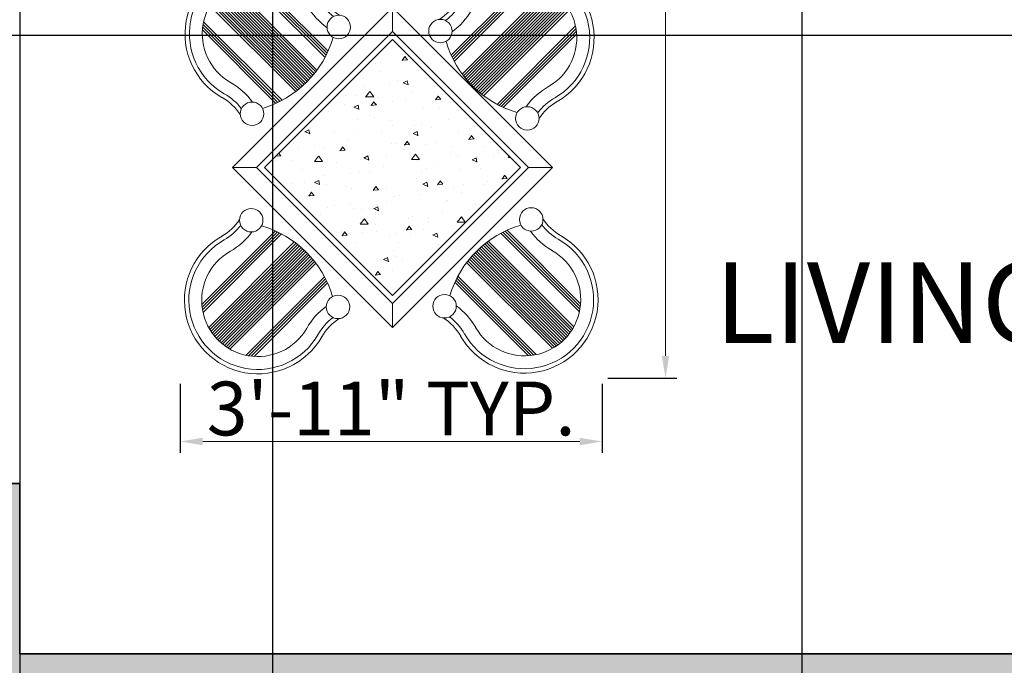
# Model space of a CAD drawing. Units: inches. Extents: x 2696 to 3240, y 1564 to 2310.
# Tile 23 of 76: x 2755 to 2864, y 1910 to 1982. Entities that reach past the tile are written whole.
import ezdxf

# ---------------------------------------------------------------- set-up
doc = ezdxf.new("R2010")
doc.units = ezdxf.units.IN
for name, color, linetype, lineweight in [('A-ANNO-DIMS', 3, 'Continuous', 18), ('A-AREA-IDEN', 7, 'Continuous', 18), ('A-FURN', 251, 'Continuous', 13), ('A-WALL', 7, 'Continuous', 35), ('A-WALL-PATT', 9, 'Continuous', 13), ('WINDOW', 2, 'Continuous', 18)]:
    doc.layers.add(name, color=color, linetype=linetype, lineweight=lineweight)
doc.styles.add('TIMES NEW', font='times.ttf')
doc.styles.add('YQ_DIM', font='SUPEROS.SHX', dxfattribs={"width": 0.8, "bigfont": 'HZDX.SHX'})
doc.dimstyles.new('Siddhuu', dxfattribs={"dimtxt": 6, "dimasz": 2.5, "dimexe": 1.25, "dimexo": 0.625, "dimtad": 1, "dimdec": 1, "dimlunit": 4, "dimtxsty": 'TIMES NEW', "dimcen": 2.5, "dimclrd": 256, "dimclre": 1, "dimclrt": 7, "dimadec": 0, "dimazin": 0, "dimtfac": 1, "dimtdec": 1, "dimtmove": 0, "dimatfit": 3, "dimfxl": 1, "dimtolj": 1, "dimlwd": -1, "dimarcsym": 0})

# ---------------------------------------------------------------- blocks, each defined once
blk = doc.blocks.new('WD_WIN4')
for p, q in [((-0.5, 0.5), (0.5, 0.5)), ((-0.5, 0.12), (0.5, 0.12)), ((-0.5, -0.12), (0.5, -0.12)), ((-0.5, -0.5), (0.5, -0.5))]:
    blk.add_line(p, q)
blk = doc.blocks.new('DINING-SET-4')
h = blk.add_hatch()
h.set_pattern_fill('AR-CONC,_O', color=256, scale=0.03156, angle=135)
h.set_pattern_definition([(185, (694.1166, -47.9622), (-3.709933, 4.421326), [0.60121, -6.613307]), (130, (694.1166, -47.962), (-3.47714, -5.050095), [0.48097, -5.290645]), (235.451, (693.8074, -47.594), (-7.187067, -0.628735), [0.51095, -5.620443]), (181.1842, (692.983, -49.096), (-5.11118, 6.98761), [0.90181, -9.91996]), (231.6356, (692.557, -48.514), (-10.81945, -0.22364), [0.76642, -8.43066]), (126.184, (692.983, -49.096), (-10.81945, -0.22362), [0.72145, -7.93597]), (156, (692.6995, -48.2457), (-1.10128, 5.66559), [0.60121, -6.613307]), (101, (692.6995, -48.2457), (-5.48951, -2.73116), [0.48097, -5.290645]), (206.4514, (692.608, -47.7735), (-6.590787, 2.93441), [0.51095, -5.620443]), (172.5, (694.1166, -47.9622), (-1.955854, -1.8180035), [0, -5.226516, 0, -5.370807, 0, -5.310686]), (142.5, (694.1166, -47.9622), (-3.726774, -0.744482), [0, -3.062161, 0, -5.106274, 0, -2.024073]), (102.5, (695.3806, -49.2263), (-2.8979947, 3.15368), [0, -2.004032, 0, -6.25258, 0, -8.296694]), (92.5, (695.9475, -49.793), (-3.873065, 2.73823), [0, -2.605242, 0, -4.152355, 0, -5.891855])])
h.paths.add_polyline_path([(23.22, 8.74), (37.5, 23.02), (23.22, 37.31), (8.94, 23.02)])
for p, q in [((15.69, 35.33), (6.93, 44.09)), ((15.81, 35.56), (7.22, 44.15)), ((15.92, 35.79), (7.52, 44.19)), ((16.03, 36.02), (7.83, 44.22)), ((14.19, 33.15), (4.42, 42.91)), ((14.34, 33.33), (4.62, 43.06)), ((14.5, 33.52), (4.82, 43.2)), ((14.65, 33.71), (5.03, 43.33)), ((14.79, 33.91), (5.25, 43.45)), ((29.77, 35.57), (37.97, 43.77)), ((29.88, 35.34), (38.28, 43.74)), ((29.99, 35.11), (38.58, 43.7)), ((30.11, 34.88), (38.86, 43.64)), ((31, 33.46), (40.55, 43.01)), ((31.15, 33.26), (40.76, 42.88)), ((13.17, 32.12), (3.39, 41.89)), ((13.35, 32.28), (3.55, 42.08)), ((13.52, 32.45), (3.71, 42.26)), ((13.69, 32.62), (3.88, 42.43)), ((13.86, 32.79), (4.05, 42.6)), ((14.03, 32.97), (4.24, 42.76)), ((31.3, 33.07), (40.97, 42.75)), ((31.45, 32.88), (41.18, 42.61)), ((31.61, 32.7), (41.37, 42.46)), ((31.77, 32.52), (41.56, 42.31)), ((31.93, 32.34), (41.74, 42.15)), ((32.1, 32.17), (41.92, 41.98)), ((32.27, 32), (42.09, 41.81)), ((12.42, 31.5), (2.84, 41.08)), ((12.61, 31.65), (2.97, 41.3)), ((12.8, 31.8), (3.1, 41.5)), ((12.99, 31.96), (3.24, 41.7)), ((23.22, 38.2), (23.22, 40.88)), ((32.45, 31.83), (42.25, 41.63)), ((32.63, 31.67), (42.4, 41.45)), ((32.81, 31.51), (42.55, 41.25)), ((32.99, 31.35), (42.69, 41.05)), ((33.18, 31.2), (42.83, 40.85)), ((33.38, 31.05), (42.96, 40.63)), ((10.44, 30.3), (2.05, 38.7)), ((10.67, 30.41), (2.09, 39)), ((10.9, 30.53), (2.15, 39.28)), ((34.9, 30.08), (43.65, 38.83)), ((35.12, 29.96), (43.7, 38.55)), ((10.21, 30.19), (2.02, 38.38)), ((35.35, 29.85), (43.75, 38.25)), ((35.58, 29.74), (43.78, 37.94)), ((8.05, 23.02), (5.37, 23.02)), ((38.4, 23.02), (41.07, 23.02)), ((10.15, 15.95), (1.95, 7.75)), ((10.38, 15.84), (1.98, 7.44)), ((10.61, 15.73), (2.02, 7.14)), ((10.84, 15.61), (2.08, 6.86)), ((35.33, 15.7), (44.08, 6.94)), ((35.55, 15.81), (44.14, 7.23)), ((35.78, 15.93), (44.18, 7.52)), ((36.01, 16.03), (44.21, 7.83)), ((12.26, 14.72), (2.71, 5.17)), ((12.46, 14.57), (2.84, 4.95)), ((12.65, 14.42), (2.97, 4.75)), ((33.33, 14.35), (43.05, 4.63)), ((33.51, 14.5), (43.19, 4.83)), ((33.7, 14.65), (43.32, 5.04)), ((33.9, 14.8), (43.45, 5.25)), ((12.83, 14.27), (3.11, 4.54)), ((13.02, 14.11), (3.26, 4.35)), ((13.2, 13.95), (3.41, 4.16)), ((13.38, 13.78), (3.57, 3.98)), ((13.55, 13.62), (3.74, 3.8)), ((13.72, 13.45), (3.91, 3.63)), ((13.89, 13.27), (4.09, 3.47)), ((32.27, 13.35), (42.07, 3.55)), ((32.44, 13.53), (42.25, 3.72)), ((32.61, 13.7), (42.42, 3.89)), ((32.78, 13.87), (42.59, 4.06)), ((32.96, 14.03), (42.75, 4.24)), ((33.14, 14.19), (42.9, 4.43)), ((14.05, 13.09), (4.27, 3.32)), ((14.21, 12.91), (4.47, 3.17)), ((14.36, 12.72), (4.67, 3.03)), ((14.52, 12.54), (4.87, 2.89)), ((14.67, 12.34), (5.08, 2.76)), ((31.49, 12.43), (41.08, 2.85)), ((31.64, 12.62), (41.29, 2.97)), ((31.8, 12.81), (41.5, 3.11)), ((31.95, 12.99), (41.69, 3.25)), ((32.11, 13.18), (41.89, 3.4)), ((15.64, 10.82), (6.89, 2.07)), ((15.75, 10.6), (7.17, 2.02)), ((15.87, 10.37), (7.47, 1.97)), ((15.98, 10.14), (7.78, 1.94)), ((30.18, 10.22), (38.38, 2.03)), ((30.29, 10.45), (38.69, 2.06)), ((30.41, 10.68), (38.99, 2.1)), ((30.52, 10.91), (39.27, 2.15)), ((23.22, 7.85), (23.22, 5.17))]:
    blk.add_line(p, q)
for points in [[(41.07, 23.02), (23.22, 40.88), (5.37, 23.02), (23.22, 5.17)], [(38.4, 23.02), (23.22, 38.2), (8.05, 23.02), (23.22, 7.85)], [(37.5, 23.02), (23.22, 37.31), (8.94, 23.02), (23.22, 8.74)]]:
    blk.add_lwpolyline(points, close=True)
for centre in [(17.23, 38.71), (28.57, 38.26), (7.55, 29.03), (38.27, 28.51), (7.46, 17.15), (38.7, 17.23), (29.03, 7.55), (17.14, 7.47)]:
    blk.add_circle(centre, 1.31)
for centre, radius, start, end in [((8.28, 37.96), 8.21, 29.1881, 240.1532), ((8.28, 37.96), 7.72, 29.1881, 240.1532), ((37.51, 37.51), 8.21, 299.8468, 150.8119), ((37.51, 37.51), 7.72, 299.8468, 150.8119), ((8.28, 37.96), 6.28, 29.2752, 240.1505), ((37.51, 37.51), 6.28, 299.8495, 150.7248), ((20.45, 44.88), 5.79, 210.1015, 236.9513), ((20.45, 44.88), 7.72, 209.8594, 234.0675), ((20.45, 44.88), 6.28, 210.1015, 232.6572), ((25.34, 44.43), 5.79, 303.0487, 329.8985), ((25.34, 44.43), 6.28, 307.3428, 329.8985), ((25.34, 44.43), 7.72, 305.9325, 330.1406), ((5.4, 40.81), 11.66, 286.5158, 343.8317), ((40.4, 40.36), 11.66, 196.1683, 253.4842), ((1.37, 25.79), 7.72, 36.1055, 60.6071), ((44.43, 25.34), 7.72, 119.3929, 143.8945), ((1.37, 25.79), 5.79, 32.6748, 60.7093), ((1.37, 25.79), 6.28, 37.2611, 60.7093), ((44.43, 25.34), 6.28, 119.2907, 142.7389), ((44.43, 25.34), 5.79, 119.2907, 147.3252), ((1.29, 20.38), 5.79, 300.1015, 326.9513), ((1.29, 20.38), 6.28, 300.1015, 322.6572), ((5.36, 5.32), 11.66, 16.5158, 73.8317), ((40.8, 5.4), 11.66, 106.1683, 163.4842), ((44.87, 20.46), 6.28, 217.3428, 239.8985), ((44.87, 20.46), 5.79, 213.0487, 239.8985), ((1.29, 20.38), 7.72, 299.8594, 324.0675), ((37.95, 8.29), 8.21, 209.8468, 60.8119), ((44.87, 20.46), 7.72, 215.9325, 240.1406), ((8.21, 8.21), 8.21, 119.1881, 330.1532), ((8.21, 8.21), 7.72, 119.1881, 330.1532), ((37.95, 8.29), 7.72, 209.8468, 60.8119), ((8.21, 8.21), 6.28, 119.2752, 330.1505), ((37.95, 8.29), 6.28, 209.8495, 60.7248), ((20.38, 1.29), 7.72, 126.1055, 150.6071), ((25.78, 1.37), 7.72, 29.3929, 53.8945), ((20.38, 1.29), 6.28, 127.2611, 150.7093), ((20.38, 1.29), 5.79, 122.6748, 150.7093), ((25.78, 1.37), 5.79, 29.2907, 57.3252), ((25.78, 1.37), 6.28, 29.2907, 52.7389)]:
    blk.add_arc(centre, radius, start, end)
blk = doc.blocks.new('*D44')
at = {"layer": 'A-ANNO-DIMS', "transparency": 16777216}
for p, q in [((2826.68, 1989.07), (2826.68, 2086.33)), ((2826.68, 1944.45), (2826.68, 1986.57))]:
    blk.add_line(p, q, dxfattribs=at)
at = {"layer": 'A-ANNO-DIMS', "color": 1, "lineweight": -2, "transparency": 16777216}
for p, q in [((2820.24, 1989.07), (2827.93, 1989.07)), ((2820.24, 1941.95), (2827.93, 1941.95))]:
    blk.add_line(p, q, dxfattribs=at)
at = {"layer": 'A-ANNO-DIMS', "transparency": 16777216}
for points in [[(2826.26, 1986.57), (2827.09, 1986.57), (2826.68, 1989.07)], [(2826.26, 1944.45), (2827.09, 1944.45), (2826.68, 1941.95)]]:
    blk.add_solid(points, dxfattribs=at)
at = {"layer": 'Defpoints', "color": 0, "transparency": 16777216}
for p in [(2819.61, 1989.07), (2826.68, 1989.07), (2819.61, 1941.95)]:
    blk.add_point(p, dxfattribs=at)
at = {"layer": 'A-ANNO-DIMS', "color": 7, "transparency": 16777216, "insert": (2822.99, 2038.95), "char_height": 6, "attachment_point": 5, "rotation": 90, "style": 'TIMES NEW'}
blk.add_mtext('\\A1;DINING SET 3\'-11" TYP.', dxfattribs=at)
blk = doc.blocks.new('*D45')
at = {"layer": 'A-ANNO-DIMS', "color": 1, "lineweight": -2, "transparency": 16777216}
for p, q in [((2772.53, 1941.33), (2772.53, 1933.64)), ((2819.61, 1941.33), (2819.61, 1933.64))]:
    blk.add_line(p, q, dxfattribs=at)
at = {"layer": 'A-ANNO-DIMS', "transparency": 16777216}
blk.add_line((2775.03, 1934.89), (2817.11, 1934.89), dxfattribs=at)
for points in [[(2775.03, 1935.3), (2775.03, 1934.47), (2772.53, 1934.89)], [(2817.11, 1935.3), (2817.11, 1934.47), (2819.61, 1934.89)]]:
    blk.add_solid(points, dxfattribs=at)
at = {"layer": 'Defpoints', "color": 0, "transparency": 16777216}
for p in [(2772.53, 1941.95), (2819.61, 1941.95), (2819.61, 1934.89)]:
    blk.add_point(p, dxfattribs=at)
at = {"layer": 'A-ANNO-DIMS', "color": 7, "transparency": 16777216, "insert": (2796.07, 1938.57), "char_height": 6, "attachment_point": 5, "style": 'TIMES NEW'}
blk.add_mtext('\\A1;3\'-11" TYP.', dxfattribs=at)
blk = doc.blocks.new('*D55')
at = {"layer": 'A-ANNO-DIMS', "color": 1, "lineweight": -2, "transparency": 16777216}
for p, q in [((3189.99, 1980.2), (2709.36, 1980.2)), ((3189.99, 1893.2), (2709.36, 1893.2))]:
    blk.add_line(p, q, dxfattribs=at)
at = {"layer": 'A-ANNO-DIMS', "transparency": 16777216}
blk.add_line((2710.61, 1895.7), (2710.61, 1977.7), dxfattribs=at)
for points in [[(2710.19, 1977.7), (2711.03, 1977.7), (2710.61, 1980.2)], [(2710.19, 1895.7), (2711.03, 1895.7), (2710.61, 1893.2)]]:
    blk.add_solid(points, dxfattribs=at)
at = {"layer": 'Defpoints', "color": 0, "transparency": 16777216}
for p in [(2710.61, 1980.2), (3190.61, 1980.2), (3190.61, 1893.2)]:
    blk.add_point(p, dxfattribs=at)
at = {"layer": 'A-ANNO-DIMS', "color": 7, "transparency": 16777216, "insert": (2706.93, 1936.7), "char_height": 6, "attachment_point": 5, "rotation": 90, "style": 'TIMES NEW'}
blk.add_mtext('\\A1;7\'-3"', dxfattribs=at)
blk = doc.blocks.new('*D57')
at = {"layer": 'A-ANNO-DIMS', "color": 1, "lineweight": -2, "transparency": 16777216}
for p, q in [((2754.61, 2018.58), (2754.61, 1568.95)), ((2956.71, 2018.58), (2956.71, 1568.95))]:
    blk.add_line(p, q, dxfattribs=at)
at = {"layer": 'A-ANNO-DIMS', "transparency": 16777216}
blk.add_line((2757.11, 1570.2), (2954.21, 1570.2), dxfattribs=at)
for points in [[(2757.11, 1570.62), (2757.11, 1569.78), (2754.61, 1570.2)], [(2954.21, 1570.62), (2954.21, 1569.78), (2956.71, 1570.2)]]:
    blk.add_solid(points, dxfattribs=at)
at = {"layer": 'Defpoints', "color": 0, "transparency": 16777216}
for p in [(2754.61, 2019.2), (2956.71, 2019.2), (2956.71, 1570.2)]:
    blk.add_point(p, dxfattribs=at)
at = {"layer": 'A-ANNO-DIMS', "color": 7, "transparency": 16777216, "insert": (2855.66, 1573.88), "char_height": 6, "attachment_point": 5, "style": 'TIMES NEW'}
blk.add_mtext('\\A1;16\'-10"', dxfattribs=at)
blk = doc.blocks.new('*D68')
at = {"layer": 'A-ANNO-DIMS', "color": 1, "lineweight": -2, "transparency": 16777216}
for p, q in [((2745.61, 2261.58), (2745.61, 1568.95)), ((2782.83, 2261.58), (2782.83, 1568.95))]:
    blk.add_line(p, q, dxfattribs=at)
at = {"layer": 'A-ANNO-DIMS', "transparency": 16777216}
blk.add_line((2748.11, 1570.2), (2780.33, 1570.2), dxfattribs=at)
for points in [[(2748.11, 1570.62), (2748.11, 1569.78), (2745.61, 1570.2)], [(2780.33, 1570.62), (2780.33, 1569.78), (2782.83, 1570.2)]]:
    blk.add_solid(points, dxfattribs=at)
at = {"layer": 'Defpoints', "color": 0, "transparency": 16777216}
for p in [(2745.61, 2262.2), (2782.83, 2262.2), (2782.83, 1570.2)]:
    blk.add_point(p, dxfattribs=at)
at = {"layer": 'A-ANNO-DIMS', "color": 7, "transparency": 16777216, "insert": (2764.22, 1573.88), "char_height": 6, "attachment_point": 5, "style": 'TIMES NEW'}
blk.add_mtext('\\A1;3\'-1"', dxfattribs=at)
blk = doc.blocks.new('*D69')
at = {"layer": 'A-ANNO-DIMS', "color": 1, "lineweight": -2, "transparency": 16777216}
for p, q in [((2841.89, 2261.58), (2841.89, 1568.95)), ((2905.91, 2261.58), (2905.91, 1568.95))]:
    blk.add_line(p, q, dxfattribs=at)
at = {"layer": 'A-ANNO-DIMS', "transparency": 16777216}
blk.add_line((2844.39, 1570.2), (2903.41, 1570.2), dxfattribs=at)
for points in [[(2844.39, 1570.62), (2844.39, 1569.78), (2841.89, 1570.2)], [(2903.41, 1570.62), (2903.41, 1569.78), (2905.91, 1570.2)]]:
    blk.add_solid(points, dxfattribs=at)
at = {"layer": 'Defpoints', "color": 0, "transparency": 16777216}
for p in [(2841.89, 2262.2), (2905.91, 2262.2), (2905.91, 1570.2)]:
    blk.add_point(p, dxfattribs=at)
at = {"layer": 'A-ANNO-DIMS', "color": 7, "transparency": 16777216, "insert": (2873.9, 1573.88), "char_height": 6, "attachment_point": 5, "style": 'TIMES NEW'}
blk.add_mtext('\\A1;5\'-4"', dxfattribs=at)
blk = doc.blocks.new('*D78')
at = {"layer": 'A-ANNO-DIMS', "transparency": 16777216}
for p, q in [((2710.61, 1901.7), (2710.61, 1935.1)), ((2710.61, 1895.7), (2710.61, 1899.2))]:
    blk.add_line(p, q, dxfattribs=at)
at = {"layer": 'A-ANNO-DIMS', "color": 1, "lineweight": -2, "transparency": 16777216}
for p, q in [((3189.99, 1901.7), (2709.36, 1901.7)), ((3189.99, 1893.2), (2709.36, 1893.2))]:
    blk.add_line(p, q, dxfattribs=at)
at = {"layer": 'A-ANNO-DIMS', "transparency": 16777216}
for points in [[(2710.19, 1899.2), (2711.03, 1899.2), (2710.61, 1901.7)], [(2710.19, 1895.7), (2711.03, 1895.7), (2710.61, 1893.2)]]:
    blk.add_solid(points, dxfattribs=at)
at = {"layer": 'Defpoints', "color": 0, "transparency": 16777216}
for p in [(2710.61, 1901.7), (3190.61, 1901.7), (3190.61, 1893.2)]:
    blk.add_point(p, dxfattribs=at)
at = {"layer": 'A-ANNO-DIMS', "color": 7, "transparency": 16777216, "insert": (2706.85, 1919.65), "char_height": 6, "attachment_point": 5, "rotation": 90, "style": 'TIMES NEW'}
blk.add_mtext('\\A1;0\'-8 1/2"', dxfattribs=at)

msp = doc.modelspace()

# ---------------------------------------------------------------- hatches: boundary and pattern name
at = {"layer": 'A-WALL-PATT', "transparency": 33554556}
h = msp.add_hatch(color=256, dxfattribs=at)
h.dxf.hatch_style = 1
h.paths.add_polyline_path([(2879.11, 2253.2), (2905.91, 2253.2), (2905.91, 2262.2), (2841.89, 2262.2), (2841.89, 2253.2), (2870.11, 2253.2), (2870.11, 2176.6), (2965.71, 2176.6), (2965.71, 2206.7), (2973.58, 2206.7), (2973.58, 2215.7), (2965.71, 2215.7), (2965.71, 2262.2), (2929.91, 2262.2), (2929.91, 2253.2), (2956.71, 2253.2), (2956.71, 2185.6), (2879.11, 2185.6)])
h.paths.add_polyline_path([(2782.83, 2262.2), (2745.61, 2262.2), (2745.61, 2228.73), (2754.61, 2228.73), (2754.61, 2253.2), (2782.83, 2253.2)])
h.paths.add_polyline_path([(2754.61, 2136.2), (2965.71, 2136.2), (2965.71, 2145.2), (2879.11, 2145.2), (2879.11, 2147.07), (2877.34, 2147.07), (2870.11, 2147.07), (2870.11, 2145.2), (2754.61, 2145.2), (2754.61, 2169.67), (2745.61, 2169.67), (2745.61, 2000.2), (2754.61, 2000.2), (2754.61, 2019.2), (2849.08, 2019.2), (2849.08, 2023.7), (2841.21, 2023.7), (2841.21, 2051.83), (2836.71, 2051.83), (2836.71, 2023.7), (2754.61, 2023.7), (2754.61, 2091.2), (2836.71, 2091.2), (2836.71, 2087.83), (2841.21, 2087.83), (2841.21, 2095.7), (2754.61, 2095.7)])
h.paths.add_polyline_path([(2965.71, 2136.2), (2956.71, 2136.2), (2956.71, 2023.7), (2885.08, 2023.7), (2885.08, 2019.2), (2956.71, 2019.2), (2956.71, 1950.58), (2965.71, 1950.58), (2965.71, 1980.2), (2973.58, 1980.2), (2973.58, 1989.2), (2965.71, 1989.2)])
h.paths.add_polyline_path([(2754.61, 1906.7), (2880.21, 1906.7), (2884.71, 1906.7), (2956.71, 1906.7), (2956.71, 1792.7), (2944.71, 1792.7), (2944.71, 1783.7), (2956.71, 1783.7), (2956.71, 1740.2), (2884.71, 1740.2), (2884.71, 1783.7), (2896.71, 1783.7), (2896.71, 1792.7), (2884.71, 1792.7), (2884.71, 1846.7), (2880.21, 1846.7), (2880.21, 1740.2), (2754.61, 1740.2), (2754.61, 1777.2), (2745.61, 1777.2), (2745.61, 1692.7), (2754.61, 1692.7), (2754.61, 1731.2), (2956.71, 1731.2), (2956.71, 1723.33), (2965.71, 1723.33), (2965.71, 1884.2), (2973.58, 1884.2), (2973.58, 1893.2), (2965.71, 1893.2), (2965.71, 1914.58), (2956.71, 1914.58), (2956.71, 1911.2), (2754.61, 1911.2), (2754.61, 1930.2), (2745.61, 1930.2), (2745.61, 1817.2), (2754.61, 1817.2), (2754.61, 1854.2), (2826.61, 1854.2), (2826.61, 1868.83), (2822.11, 1868.83), (2822.11, 1858.7), (2754.61, 1858.7)])
h.paths.add_polyline_path([(2965.71, 1656.2), (3008.24, 1656.2), (3008.24, 1665.2), (2965.71, 1665.2), (2965.71, 1693.33), (2956.71, 1693.33), (2956.71, 1686.2), (2934.58, 1686.2), (2934.58, 1681.7), (2956.71, 1681.7), (2956.71, 1614.2), (2896.71, 1614.2), (2896.71, 1681.7), (2904.58, 1681.7), (2904.58, 1686.2), (2892.21, 1686.2), (2892.21, 1614.2), (2858.41, 1614.2), (2858.41, 1605.2), (2965.71, 1605.2)])
h.paths.add_polyline_path([(2788.41, 1614.2), (2754.61, 1614.2), (2754.61, 1652.7), (2745.61, 1652.7), (2745.61, 1605.2), (2788.41, 1605.2)])
h.paths.add_polyline_path([(3199.61, 1633.05), (3190.61, 1633.05), (3190.61, 1614.2), (3082.61, 1614.2), (3082.61, 1665.2), (3070.24, 1665.2), (3070.24, 1656.2), (3078.11, 1656.2), (3078.11, 1605.2), (3199.61, 1605.2)])
h.paths.add_polyline_path([(3199.61, 1702.05), (3190.61, 1702.05), (3190.61, 1699.7), (3106.61, 1699.7), (3106.61, 1747.7), (3190.61, 1747.7), (3190.61, 1752.2), (3082.61, 1752.2), (3082.61, 1760.08), (3078.11, 1760.08), (3078.11, 1747.7), (3102.11, 1747.7), (3102.11, 1699.7), (3078.11, 1699.7), (3078.11, 1695.2), (3190.61, 1695.2), (3190.61, 1676.35), (3199.61, 1676.35)])
h.paths.add_polyline_path([(3199.61, 1783.2), (3190.61, 1783.2), (3190.61, 1745.35), (3199.61, 1745.35)])
h.paths.add_polyline_path([(3082.61, 1884.2), (3190.61, 1884.2), (3190.61, 1853.2), (3199.61, 1853.2), (3199.61, 1901.7), (3190.61, 1901.7), (3190.61, 1893.2), (3005.58, 1893.2), (3005.58, 1891.28), (3005.58, 1884.2), (3078.11, 1884.2), (3078.11, 1792.08), (3082.61, 1792.08)])
h.paths.add_polyline_path([(3199.61, 1994.7), (3190.61, 1994.7), (3190.61, 1989.2), (3073.71, 1989.2), (3073.71, 2034.2), (3069.21, 2034.2), (3069.21, 1989.2), (3005.58, 1989.2), (3005.58, 1980.2), (3190.61, 1980.2), (3190.61, 1971.7), (3199.61, 1971.7)])
h.paths.add_polyline_path([(3199.61, 2155.2), (3190.61, 2155.2), (3190.61, 2064.7), (3199.61, 2064.7)])
h.paths.add_polyline_path([(3190.61, 2074.7), (3106.61, 2074.7), (3106.61, 2122.7), (3190.61, 2122.7), (3190.61, 2127.2), (3082.71, 2127.2), (3082.71, 2135.08), (3073.71, 2135.08), (3073.71, 2122.7), (3102.11, 2122.7), (3102.11, 2074.7), (3069.21, 2074.7), (3069.21, 2070.2), (3190.61, 2070.2)])
h.paths.add_polyline_path([(3082.71, 2253.2), (3190.61, 2253.2), (3190.61, 2225.2), (3199.61, 2225.2), (3199.61, 2262.2), (3073.71, 2262.2), (3073.71, 2215.7), (3035.58, 2215.7), (3035.58, 2206.7), (3073.71, 2206.7), (3073.71, 2171.08), (3082.71, 2171.08)])

# ---------------------------------------------------------------- linework, layer by layer
at = {"layer": 'A-WALL'}
for p, q in [((2754.61, 1930.2), (2745.61, 1930.2)), ((2754.61, 1911.2), (2754.61, 1930.2)), ((2754.61, 1911.2), (2956.71, 1911.2))]:
    msp.add_line(p, q, dxfattribs=at)

# ---------------------------------------------------------------- block references
at = {"layer": 'A-FURN'}
msp.add_blockref('DINING-SET-4', (2772.99, 1942.44), dxfattribs=at)
at = {"layer": 'WINDOW', "xscale": 70, "yscale": 8.999999999999545, "zscale": 70, "rotation": 270}
msp.add_blockref('WD_WIN4', (2750.11, 1965.2), dxfattribs=at)

# ---------------------------------------------------------------- texts
at = {"layer": 'A-AREA-IDEN', "insert": (2832.18, 1954.9), "char_height": 9, "attachment_point": 1, "style": 'YQ_DIM'}
msp.add_mtext_dynamic_manual_height_columns('LIVING/DINING', width=92.6128, gutter_width=12.5, heights=[0], dxfattribs=at)

# ---------------------------------------------------------------- dimensions: what is measured, and where the dimension line sits
at = {"layer": 'A-ANNO-DIMS'}
for base, p1, p2, picture, middle in [((2782.83, 1570.2), (2745.61, 2262.2), (2782.83, 2262.2), '*D68', (2764.22, 1573.88)), ((2905.91, 1570.2), (2841.89, 2262.2), (2905.91, 2262.2), '*D69', (2873.9, 1573.88)), ((2956.71, 1570.2), (2754.61, 2019.2), (2956.71, 2019.2), '*D57', (2855.66, 1573.88))]:
    dim = msp.add_linear_dim(base=base, p1=p1, p2=p2, dimstyle='Siddhuu', override={"dimdec": 1, "dimlfac": 1, "dimrnd": 0, "dimzin": 1, "dimdsep": 46, "dimlunit": 4, "dimfrac": 2}, dxfattribs=at)
    dim.commit()
    dim.dimension.update_dxf_attribs({"geometry": picture, "text_midpoint": middle})
dim = msp.add_linear_dim(base=(2826.68, 1989.07), p1=(2819.61, 1941.95), p2=(2819.61, 1989.07), angle=90, text='DINING SET <> TYP.', dimstyle='Siddhuu', override={"dimdec": 1, "dimlfac": 1, "dimrnd": 0, "dimzin": 1, "dimdsep": 46, "dimlunit": 4, "dimfrac": 2}, dxfattribs=at)
dim.commit()
dim.dimension.update_dxf_attribs({"geometry": '*D44', "text_midpoint": (2822.99, 2038.95)})
for base, p2, picture, middle in [((2710.61, 1980.2), (3190.61, 1980.2), '*D55', (2706.93, 1936.7)), ((2710.61, 1901.7), (3190.61, 1901.7), '*D78', (2706.85, 1919.65))]:
    dim = msp.add_linear_dim(base=base, p1=(3190.61, 1893.2), p2=p2, angle=90, dimstyle='Siddhuu', override={"dimdec": 1, "dimlfac": 1, "dimrnd": 0, "dimzin": 1, "dimdsep": 46, "dimlunit": 4, "dimfrac": 2}, dxfattribs=at)
    dim.commit()
    dim.dimension.update_dxf_attribs({"geometry": picture, "text_midpoint": middle})
dim = msp.add_linear_dim(base=(2819.61, 1934.89), p1=(2772.53, 1941.95), p2=(2819.61, 1941.95), text='<> TYP.', dimstyle='Siddhuu', override={"dimdec": 1, "dimlfac": 1, "dimrnd": 0, "dimzin": 1, "dimdsep": 46, "dimlunit": 4, "dimfrac": 2}, dxfattribs=at)
dim.commit()
dim.dimension.update_dxf_attribs({"geometry": '*D45', "text_midpoint": (2796.07, 1938.57)})

doc.saveas('drawing.dxf')
